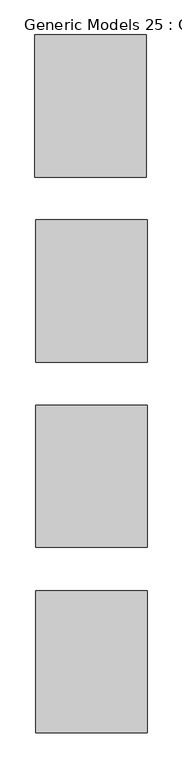
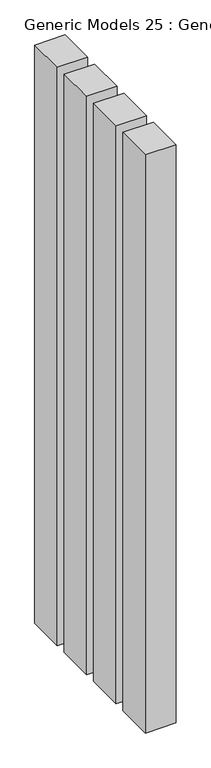
"""IFC4 building model written with IfcOpenShell, lengths in millimetres: proxy geometry, Generic Models 25 : Generic Models 25."""

from ifc_helpers import new_model, si_unit, frame, origin, place, context, project, spatial, polyline, outline, extrude, source, transform, mapped, element, save


def generic_models_25_generic_models_25_fd65dc18(model_context):
    return source(origin(), model_context, "Body", "SweptSolid", [
        extrude(outline(polyline([(66.1413992, -682.3505702), (370.9413992, -682.3505702), (370.9413992, -1072.0753999), (66.1413992, -1072.0753999), (66.1413992, -682.3505702)])), frame((0.0, 0.0, 304.8), z_axis=(0.0, 0.0, 1.0), x_axis=(1.0, 0.0, 0.0)), (0.0, 0.0, 1.0), 6107.811293),
        extrude(outline(polyline([(66.1413992, -174.3505702), (370.9413992, -174.3505702), (370.9413992, -564.0753999), (66.1413992, -564.0753999), (66.1413992, -174.3505702)])), frame((0.0, 0.0, 304.8), z_axis=(0.0, 0.0, 1.0), x_axis=(1.0, 0.0, 0.0)), (0.0, 0.0, 1.0), 6107.811293),
        extrude(outline(polyline([(66.1413992, 333.6494298), (370.9413992, 333.6494298), (370.9413992, -56.0753999), (66.1413992, -56.0753999), (66.1413992, 333.6494298)])), frame((0.0, 0.0, 304.8), z_axis=(0.0, 0.0, 1.0), x_axis=(1.0, 0.0, 0.0)), (0.0, 0.0, 1.0), 6107.811293),
        extrude(outline(polyline([(63.4776879, 840.4119673), (368.2776879, 840.4119673), (368.2776879, 450.6871377), (63.4776879, 450.6871377), (63.4776879, 840.4119673)])), frame((0.0, 0.0, 304.8), z_axis=(0.0, 0.0, 1.0), x_axis=(1.0, 0.0, 0.0)), (0.0, 0.0, 1.0), 6107.811293),
    ])


if __name__ == "__main__":
    model = new_model("IFC4")
    model_context = context("Model", 3, world=origin())
    ifc_project = project(units=[si_unit("LENGTHUNIT", "METRE", prefix="MILLI")], contexts=[model_context])
    site = spatial("IfcSite", under=ifc_project)
    building = spatial("IfcBuilding", under=site)
    placement = place(None, origin())
    generic_models_25_generic_models_25_shape = generic_models_25_generic_models_25_fd65dc18(model_context)
    element("IfcBuildingElementProxy", 1, Name="Generic Models 25 : Generic Models 25", ObjectType="Generic Models 25 : Generic Models 25", at=placement, inside=building, context=model_context, shape_type="MappedRepresentation", body=[
        mapped(generic_models_25_generic_models_25_shape, transform((0.0, 0.0, 0.0), x_axis=(1.0, 0.0, 0.0), y_axis=(0.0, 1.0, 0.0), z_axis=(0.0, 0.0, 1.0))),
    ])
    save(model, "model.ifc")

# Revit data of these elements
# Element 1 (IfcBuildingElementProxy, "Generic Models 25 : Generic Models 25")
#   Materials on its faces: "feature frame"
# Materials
#   "feature frame": class "Generic", colour RGB 120 120 120, transparency 0, Cost = 0
